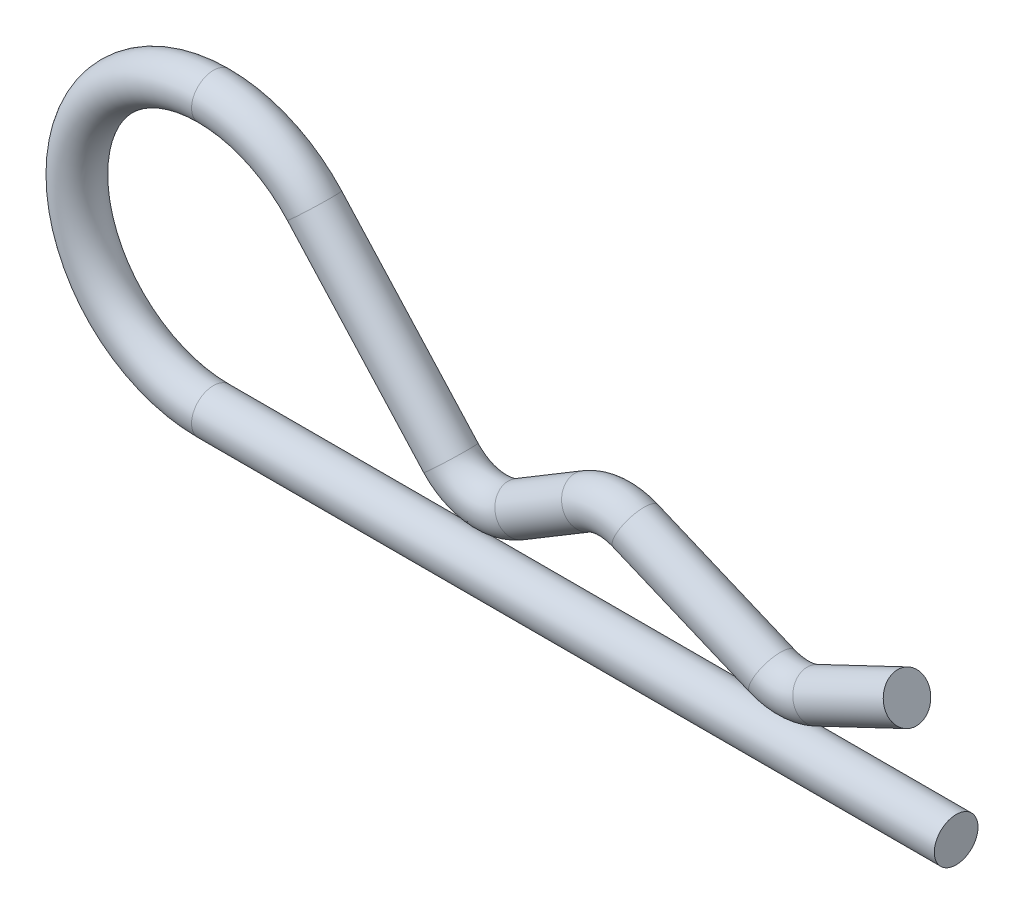
ISO-10303-21;
HEADER;
FILE_DESCRIPTION(('STEP AP214'),'2;1');
FILE_NAME('part.step','',(''),(''),'','','');
FILE_SCHEMA(('AUTOMOTIVE_DESIGN { 1 0 10303 214 1 1 1 1 }'));
ENDSEC;
DATA;
#1=APPLICATION_CONTEXT('core data for automotive mechanical design processes');
#2=APPLICATION_PROTOCOL_DEFINITION('international standard','automotive_design',2000,#1);
#3=PRODUCT_CONTEXT('',#1,'mechanical');
#4=PRODUCT('Part','Part','',(#3));
#5=PRODUCT_RELATED_PRODUCT_CATEGORY('part','',(#4));
#6=PRODUCT_DEFINITION_FORMATION('','',#4);
#7=PRODUCT_DEFINITION_CONTEXT('part definition',#1,'design');
#8=PRODUCT_DEFINITION('design','',#6,#7);
#9=PRODUCT_DEFINITION_SHAPE('','',#8);
#10=(LENGTH_UNIT() NAMED_UNIT(*) SI_UNIT(.MILLI.,.METRE.));
#11=(NAMED_UNIT(*) PLANE_ANGLE_UNIT() SI_UNIT($,.RADIAN.));
#12=(NAMED_UNIT(*) SI_UNIT($,.STERADIAN.) SOLID_ANGLE_UNIT());
#13=UNCERTAINTY_MEASURE_WITH_UNIT(LENGTH_MEASURE(1.E-05),#10,'distance_accuracy_value','');
#14=(GEOMETRIC_REPRESENTATION_CONTEXT(3) GLOBAL_UNCERTAINTY_ASSIGNED_CONTEXT((#13)) GLOBAL_UNIT_ASSIGNED_CONTEXT((#10,
#11,#12)) REPRESENTATION_CONTEXT('',''));
#15=CARTESIAN_POINT('',(0.,0.,0.));
#16=DIRECTION('',(0.,0.,1.));
#17=DIRECTION('',(1.,0.,0.));
#18=AXIS2_PLACEMENT_3D('',#15,#16,#17);
#19=CARTESIAN_POINT('',(0.,0.,0.));
#20=DIRECTION('',(1.,0.,0.));
#21=DIRECTION('',(0.,1.,0.));
#22=AXIS2_PLACEMENT_3D('',#19,#20,#21);
#23=PLANE('',#22);
#24=CARTESIAN_POINT('',(0.,0.,0.));
#25=DIRECTION('',(1.,0.,0.));
#26=DIRECTION('',(0.,1.,0.));
#27=AXIS2_PLACEMENT_3D('',#24,#25,#26);
#28=CIRCLE('',#27,2.);
#29=CARTESIAN_POINT('',(0.,2.,0.));
#30=VERTEX_POINT('',#29);
#31=EDGE_CURVE('E86',#30,#30,#28,.T.);
#32=ORIENTED_EDGE('',*,*,#31,.T.);
#33=EDGE_LOOP('',(#32));
#34=FACE_BOUND('',#33,.T.);
#35=ADVANCED_FACE('F47',(#34),#23,.T.);
#36=CARTESIAN_POINT('',(-4.50000000000001,9.,0.));
#37=DIRECTION('',(-0.902990579928772,-0.429660345575316,0.));
#38=DIRECTION('',(0.429660345575316,-0.902990579928772,0.));
#39=AXIS2_PLACEMENT_3D('',#36,#37,#38);
#40=PLANE('',#39);
#41=CARTESIAN_POINT('',(-4.50000000000001,9.,0.));
#42=DIRECTION('',(-0.902990579928772,-0.429660345575316,0.));
#43=DIRECTION('',(0.429660345575316,-0.902990579928772,0.));
#44=AXIS2_PLACEMENT_3D('',#41,#42,#43);
#45=CIRCLE('',#44,2.);
#46=CARTESIAN_POINT('',(-3.64067930884937,7.19401884014245,0.));
#47=VERTEX_POINT('',#46);
#48=EDGE_CURVE('E11',#47,#47,#45,.T.);
#49=ORIENTED_EDGE('',*,*,#48,.F.);
#50=EDGE_LOOP('',(#49));
#51=FACE_BOUND('',#50,.T.);
#52=ADVANCED_FACE('F92',(#51),#40,.F.);
#53=CARTESIAN_POINT('',(0.,0.,0.));
#54=DIRECTION('',(-1.,0.,0.));
#55=DIRECTION('',(0.,-1.,0.));
#56=AXIS2_PLACEMENT_3D('',#53,#54,#55);
#57=CYLINDRICAL_SURFACE('',#56,2.);
#58=CARTESIAN_POINT('',(-68.,0.,0.));
#59=DIRECTION('',(1.,0.,0.));
#60=DIRECTION('',(0.,1.,0.));
#61=AXIS2_PLACEMENT_3D('',#58,#59,#60);
#62=CIRCLE('',#61,2.);
#63=CARTESIAN_POINT('',(-68.,-2.00000000000001,0.));
#64=VERTEX_POINT('',#63);
#65=EDGE_CURVE('E81',#64,#64,#62,.T.);
#66=ORIENTED_EDGE('',*,*,#65,.T.);
#67=EDGE_LOOP('',(#66));
#68=FACE_BOUND('',#67,.T.);
#69=ORIENTED_EDGE('',*,*,#31,.F.);
#70=EDGE_LOOP('',(#69));
#71=FACE_BOUND('',#70,.T.);
#72=ADVANCED_FACE('F91',(#68,#71),#57,.T.);
#73=CARTESIAN_POINT('',(-68.,12.5,0.));
#74=DIRECTION('',(0.,0.,-1.));
#75=DIRECTION('',(-1.,0.,0.));
#76=AXIS2_PLACEMENT_3D('',#73,#74,#75);
#77=TOROIDAL_SURFACE('',#76,12.5,2.);
#78=CARTESIAN_POINT('',(-68.,25.,0.));
#79=DIRECTION('',(-1.,0.,0.));
#80=DIRECTION('',(0.,-1.,0.));
#81=AXIS2_PLACEMENT_3D('',#78,#79,#80);
#82=CIRCLE('',#81,2.);
#83=CARTESIAN_POINT('',(-68.,27.,0.));
#84=VERTEX_POINT('',#83);
#85=EDGE_CURVE('E79',#84,#84,#82,.T.);
#86=CARTESIAN_POINT('',(-68.,12.5,0.));
#87=DIRECTION('',(0.,0.,-1.));
#88=DIRECTION('',(-1.,0.,0.));
#89=AXIS2_PLACEMENT_3D('',#86,#87,#88);
#90=CIRCLE('',#89,14.5);
#91=EDGE_CURVE('',#64,#84,#90,.T.);
#92=ORIENTED_EDGE('',*,*,#65,.F.);
#93=ORIENTED_EDGE('',*,*,#85,.T.);
#94=ORIENTED_EDGE('',*,*,#91,.T.);
#95=ORIENTED_EDGE('',*,*,#91,.F.);
#96=EDGE_LOOP('',(#92,#94,#93,#95));
#97=FACE_BOUND('',#96,.T.);
#98=ADVANCED_FACE('F93',(#97),#77,.T.);
#99=CARTESIAN_POINT('',(-68.,12.5,0.));
#100=DIRECTION('',(0.,0.,-1.));
#101=DIRECTION('',(-1.,0.,0.));
#102=AXIS2_PLACEMENT_3D('',#99,#100,#101);
#103=TOROIDAL_SURFACE('',#102,12.5,2.);
#104=CARTESIAN_POINT('',(-58.7423968628985,20.8992133057762,0.));
#105=DIRECTION('',(-0.671937064462097,0.740608250968121,0.));
#106=DIRECTION('',(-0.740608250968121,-0.671937064462098,0.));
#107=AXIS2_PLACEMENT_3D('',#104,#105,#106);
#108=CIRCLE('',#107,2.);
#109=CARTESIAN_POINT('',(-57.2611803609622,22.2430874347004,0.));
#110=VERTEX_POINT('',#109);
#111=EDGE_CURVE('E77',#110,#110,#108,.T.);
#112=CARTESIAN_POINT('',(-68.,12.5,0.));
#113=DIRECTION('',(0.,0.,-1.));
#114=DIRECTION('',(-1.,0.,0.));
#115=AXIS2_PLACEMENT_3D('',#112,#113,#114);
#116=CIRCLE('',#115,14.5);
#117=EDGE_CURVE('',#84,#110,#116,.T.);
#118=ORIENTED_EDGE('',*,*,#85,.F.);
#119=ORIENTED_EDGE('',*,*,#111,.T.);
#120=ORIENTED_EDGE('',*,*,#117,.T.);
#121=ORIENTED_EDGE('',*,*,#117,.F.);
#122=EDGE_LOOP('',(#118,#120,#119,#121));
#123=FACE_BOUND('',#122,.T.);
#124=ADVANCED_FACE('F102',(#123),#103,.T.);
#125=CARTESIAN_POINT('',(-58.7423968628985,20.8992133057762,0.));
#126=DIRECTION('',(0.671937064462097,-0.740608250968121,0.));
#127=DIRECTION('',(0.740608250968121,0.671937064462097,0.));
#128=AXIS2_PLACEMENT_3D('',#125,#126,#127);
#129=CYLINDRICAL_SURFACE('',#128,2.);
#130=CARTESIAN_POINT('',(-46.2592602757717,7.14031467768951,0.));
#131=DIRECTION('',(-0.671937064462097,0.740608250968121,0.));
#132=DIRECTION('',(-0.740608250968122,-0.671937064462097,0.));
#133=AXIS2_PLACEMENT_3D('',#130,#131,#132);
#134=CIRCLE('',#133,2.);
#135=CARTESIAN_POINT('',(-47.7404767777079,5.79644054876531,0.));
#136=VERTEX_POINT('',#135);
#137=EDGE_CURVE('E71',#136,#136,#134,.T.);
#138=ORIENTED_EDGE('',*,*,#137,.T.);
#139=EDGE_LOOP('',(#138));
#140=FACE_BOUND('',#139,.T.);
#141=ORIENTED_EDGE('',*,*,#111,.F.);
#142=EDGE_LOOP('',(#141));
#143=FACE_BOUND('',#142,.T.);
#144=ADVANCED_FACE('F127',(#140,#143),#129,.T.);
#145=CARTESIAN_POINT('',(-42.5562190209311,10.5,0.));
#146=DIRECTION('',(0.,0.,1.));
#147=DIRECTION('',(1.,0.,0.));
#148=AXIS2_PLACEMENT_3D('',#145,#146,#147);
#149=TOROIDAL_SURFACE('',#148,5.,2.);
#150=CARTESIAN_POINT('',(-39.9804104566553,6.214535003036,0.));
#151=DIRECTION('',(-0.857092999392798,-0.515161712855155,0.));
#152=DIRECTION('',(0.515161712855155,-0.857092999392798,0.));
#153=AXIS2_PLACEMENT_3D('',#150,#151,#152);
#154=CIRCLE('',#153,2.);
#155=CARTESIAN_POINT('',(-38.950087030945,4.50034900425041,0.));
#156=VERTEX_POINT('',#155);
#157=EDGE_CURVE('E72',#156,#156,#154,.T.);
#158=CARTESIAN_POINT('',(-42.5562190209311,10.5,0.));
#159=DIRECTION('',(0.,0.,1.));
#160=DIRECTION('',(1.,0.,0.));
#161=AXIS2_PLACEMENT_3D('',#158,#159,#160);
#162=CIRCLE('',#161,7.);
#163=EDGE_CURVE('',#136,#156,#162,.T.);
#164=ORIENTED_EDGE('',*,*,#137,.F.);
#165=ORIENTED_EDGE('',*,*,#157,.T.);
#166=ORIENTED_EDGE('',*,*,#163,.T.);
#167=ORIENTED_EDGE('',*,*,#163,.F.);
#168=EDGE_LOOP('',(#164,#166,#165,#167));
#169=FACE_BOUND('',#168,.T.);
#170=ADVANCED_FACE('F128',(#169),#149,.T.);
#171=CARTESIAN_POINT('',(-39.9804104566553,6.214535003036,0.));
#172=DIRECTION('',(0.857092999392798,0.515161712855156,0.));
#173=DIRECTION('',(-0.515161712855156,0.857092999392798,0.));
#174=AXIS2_PLACEMENT_3D('',#171,#172,#173);
#175=CYLINDRICAL_SURFACE('',#174,2.);
#176=CARTESIAN_POINT('',(-33.8729527001016,9.88546499696399,0.));
#177=DIRECTION('',(-0.857092999392798,-0.515161712855156,0.));
#178=DIRECTION('',(0.515161712855156,-0.857092999392798,0.));
#179=AXIS2_PLACEMENT_3D('',#176,#177,#178);
#180=CIRCLE('',#179,2.);
#181=CARTESIAN_POINT('',(-34.9032761258119,11.5996509957496,0.));
#182=VERTEX_POINT('',#181);
#183=EDGE_CURVE('E66',#182,#182,#180,.T.);
#184=ORIENTED_EDGE('',*,*,#183,.T.);
#185=EDGE_LOOP('',(#184));
#186=FACE_BOUND('',#185,.T.);
#187=ORIENTED_EDGE('',*,*,#157,.F.);
#188=EDGE_LOOP('',(#187));
#189=FACE_BOUND('',#188,.T.);
#190=ADVANCED_FACE('F122',(#186,#189),#175,.T.);
#191=CARTESIAN_POINT('',(-31.2971441358258,5.6,0.));
#192=DIRECTION('',(0.,0.,-1.));
#193=DIRECTION('',(-1.,0.,0.));
#194=AXIS2_PLACEMENT_3D('',#191,#192,#193);
#195=TOROIDAL_SURFACE('',#194,5.,2.);
#196=CARTESIAN_POINT('',(-29.3622637039336,10.2104487541107,0.));
#197=DIRECTION('',(-0.922089750822139,0.38697608637843,0.));
#198=DIRECTION('',(-0.38697608637843,-0.922089750822139,0.));
#199=AXIS2_PLACEMENT_3D('',#196,#197,#198);
#200=CIRCLE('',#199,2.);
#201=CARTESIAN_POINT('',(-28.5883115311768,12.054628255755,0.));
#202=VERTEX_POINT('',#201);
#203=EDGE_CURVE('E65',#202,#202,#200,.T.);
#204=CARTESIAN_POINT('',(-31.2971441358258,5.6,0.));
#205=DIRECTION('',(0.,0.,-1.));
#206=DIRECTION('',(-1.,0.,0.));
#207=AXIS2_PLACEMENT_3D('',#204,#205,#206);
#208=CIRCLE('',#207,7.);
#209=EDGE_CURVE('',#182,#202,#208,.T.);
#210=ORIENTED_EDGE('',*,*,#183,.F.);
#211=ORIENTED_EDGE('',*,*,#203,.T.);
#212=ORIENTED_EDGE('',*,*,#209,.T.);
#213=ORIENTED_EDGE('',*,*,#209,.F.);
#214=EDGE_LOOP('',(#210,#212,#211,#213));
#215=FACE_BOUND('',#214,.T.);
#216=ADVANCED_FACE('F120',(#215),#195,.T.);
#217=CARTESIAN_POINT('',(-29.3622637039336,10.2104487541107,0.));
#218=DIRECTION('',(0.922089750822139,-0.38697608637843,0.));
#219=DIRECTION('',(0.38697608637843,0.922089750822139,0.));
#220=AXIS2_PLACEMENT_3D('',#217,#218,#219);
#221=CYLINDRICAL_SURFACE('',#220,2.);
#222=CARTESIAN_POINT('',(-16.8629560007989,4.96482795300513,0.));
#223=DIRECTION('',(-0.922089750822139,0.38697608637843,0.));
#224=DIRECTION('',(-0.38697608637843,-0.922089750822139,0.));
#225=AXIS2_PLACEMENT_3D('',#222,#223,#224);
#226=CIRCLE('',#225,2.);
#227=CARTESIAN_POINT('',(-17.6369081735557,3.12064845136085,0.));
#228=VERTEX_POINT('',#227);
#229=EDGE_CURVE('E56',#228,#228,#226,.T.);
#230=ORIENTED_EDGE('',*,*,#229,.T.);
#231=EDGE_LOOP('',(#230));
#232=FACE_BOUND('',#231,.T.);
#233=ORIENTED_EDGE('',*,*,#203,.F.);
#234=EDGE_LOOP('',(#233));
#235=FACE_BOUND('',#234,.T.);
#236=ADVANCED_FACE('F115',(#232,#235),#221,.T.);
#237=CARTESIAN_POINT('',(-14.9280755689067,9.57527670711582,0.));
#238=DIRECTION('',(0.,0.,1.));
#239=DIRECTION('',(1.,0.,0.));
#240=AXIS2_PLACEMENT_3D('',#237,#238,#239);
#241=TOROIDAL_SURFACE('',#240,5.,2.);
#242=CARTESIAN_POINT('',(-12.7797738410301,5.06032380747197,0.));
#243=DIRECTION('',(-0.902990579928772,-0.429660345575316,0.));
#244=DIRECTION('',(0.429660345575316,-0.902990579928772,0.));
#245=AXIS2_PLACEMENT_3D('',#242,#243,#244);
#246=CIRCLE('',#245,2.);
#247=CARTESIAN_POINT('',(-11.9204531498795,3.25434264761443,0.));
#248=VERTEX_POINT('',#247);
#249=EDGE_CURVE('E54',#248,#248,#246,.T.);
#250=CARTESIAN_POINT('',(-14.9280755689067,9.57527670711582,0.));
#251=DIRECTION('',(0.,0.,1.));
#252=DIRECTION('',(1.,0.,0.));
#253=AXIS2_PLACEMENT_3D('',#250,#251,#252);
#254=CIRCLE('',#253,7.);
#255=EDGE_CURVE('',#228,#248,#254,.T.);
#256=ORIENTED_EDGE('',*,*,#229,.F.);
#257=ORIENTED_EDGE('',*,*,#249,.T.);
#258=ORIENTED_EDGE('',*,*,#255,.T.);
#259=ORIENTED_EDGE('',*,*,#255,.F.);
#260=EDGE_LOOP('',(#256,#258,#257,#259));
#261=FACE_BOUND('',#260,.T.);
#262=ADVANCED_FACE('F109',(#261),#241,.T.);
#263=CARTESIAN_POINT('',(-12.7797738410301,5.06032380747196,0.));
#264=DIRECTION('',(0.902990579928772,0.429660345575316,0.));
#265=DIRECTION('',(-0.429660345575316,0.902990579928772,0.));
#266=AXIS2_PLACEMENT_3D('',#263,#264,#265);
#267=CYLINDRICAL_SURFACE('',#266,2.);
#268=ORIENTED_EDGE('',*,*,#48,.T.);
#269=EDGE_LOOP('',(#268));
#270=FACE_BOUND('',#269,.T.);
#271=ORIENTED_EDGE('',*,*,#249,.F.);
#272=EDGE_LOOP('',(#271));
#273=FACE_BOUND('',#272,.T.);
#274=ADVANCED_FACE('F103',(#270,#273),#267,.T.);
#275=CLOSED_SHELL('',(#35,#52,#72,#98,#124,#144,#170,#190,#216,#236,#262,#274));
#276=MANIFOLD_SOLID_BREP('B2',#275);
#277=ADVANCED_BREP_SHAPE_REPRESENTATION('',(#18,#276),#14);
#278=SHAPE_DEFINITION_REPRESENTATION(#9,#277);
ENDSEC;
END-ISO-10303-21;
